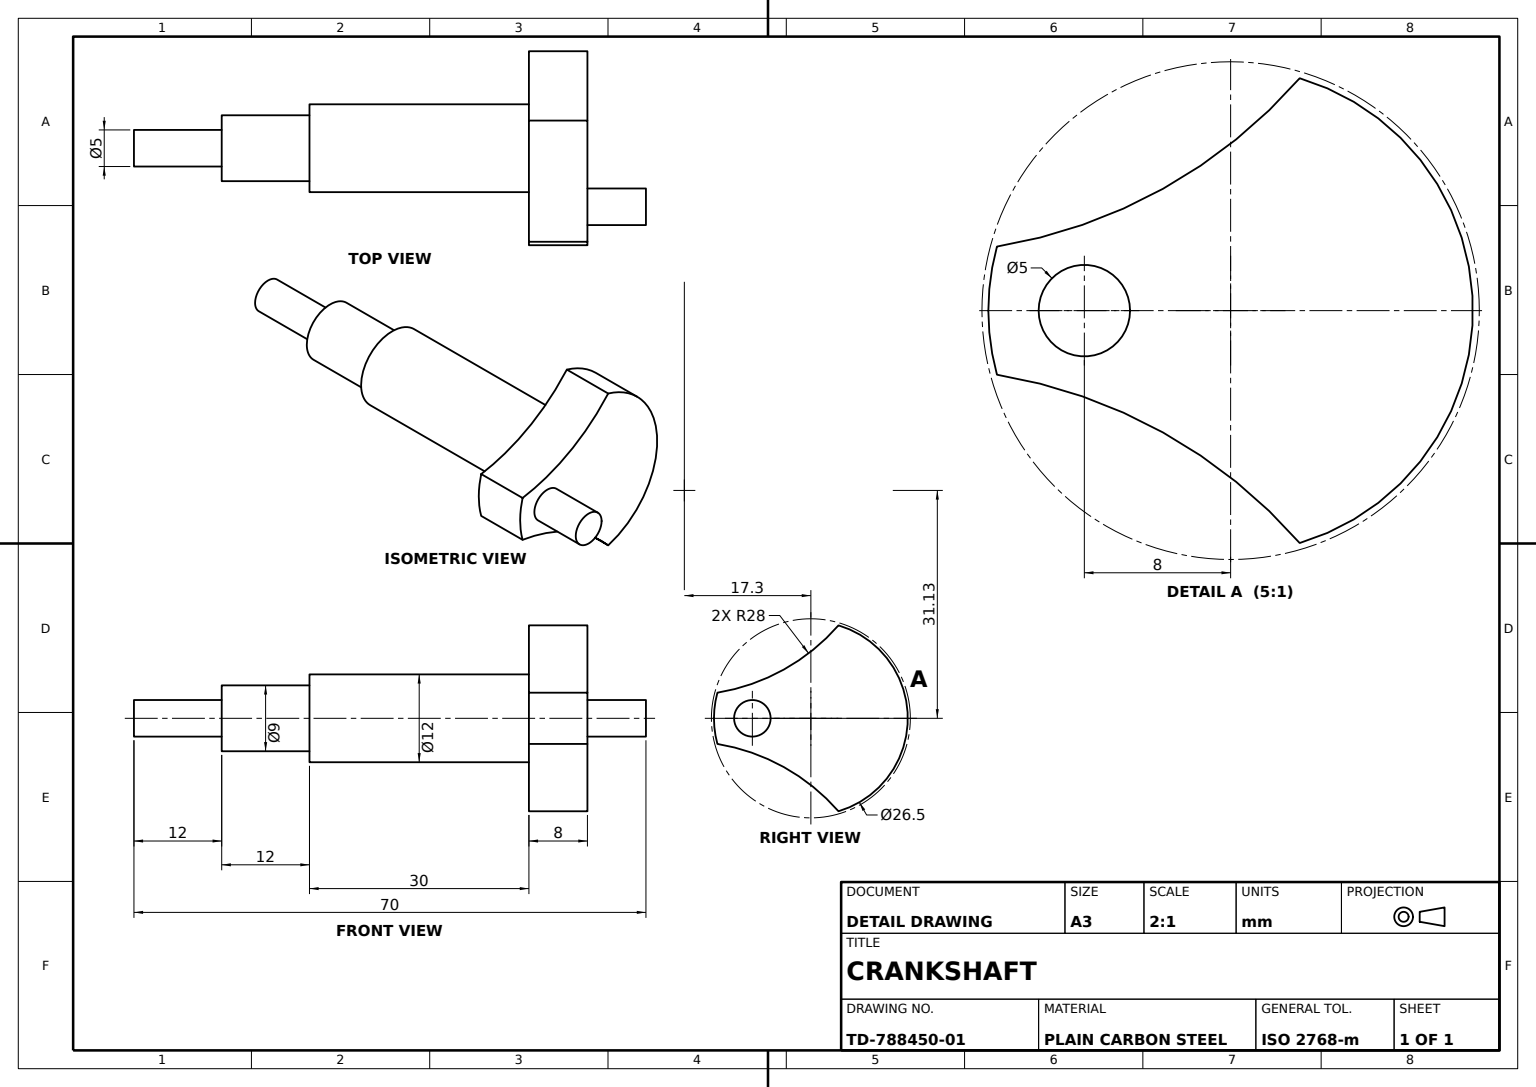
from build123d import *

# Parameters (mm, degrees)
MAIN_JOURNAL_PROFILE_12_R = 6
MAIN_JOURNAL_12_DEPTH     = 30
STEP_JOURNAL_PROFILE_9_R  = 4.5
STEP_JOURNAL_9_DEPTH      = 12
SHAFT_END_PROFILE_5_R     = 2.5
SHAFT_END_5_DEPTH         = 12
CRANK_WEB_DEPTH           = 8
CRANK_PIN_PROFILE_R       = 2.5
CRANK_PIN_DEPTH           = 8


with BuildPart() as part:
    # Main Journal Profile Ø12 → Main Journal Ø12 (new body)
    with BuildSketch(Plane.XY):
        Circle(MAIN_JOURNAL_PROFILE_12_R)
    extrude(amount=MAIN_JOURNAL_12_DEPTH)

    # Step Journal Profile Ø9 → Step Journal Ø9 (add)
    with BuildSketch(Plane.XY.offset(30)):
        Circle(STEP_JOURNAL_PROFILE_9_R)
    extrude(amount=STEP_JOURNAL_9_DEPTH)

    # Shaft End Profile Ø5 → Shaft End Ø5 (add)
    with BuildSketch(Plane.XY.offset(42)):
        Circle(SHAFT_END_PROFILE_5_R)
    extrude(amount=SHAFT_END_5_DEPTH)

    # Crank Web Profile → Crank Web (add)
    with BuildSketch(Plane(origin=(0, 0, 0), x_dir=(-1, 0, 0), z_dir=(0, 0, -1))):
        with BuildLine():
            ThreePointArc((-12.779377919, 3.5), (-13.25, 0), (-12.779377919, -3.5))
            ThreePointArc((-12.779377919, -3.5), (-3.699194839, -6.657412557), (3.777827997, -12.7000203))
            ThreePointArc((3.777827997, -12.7000203), (13.25, 0), (3.777827997, 12.7000203))
            ThreePointArc((3.777827997, 12.7000203), (-3.699194839, 6.657412557), (-12.779377919, 3.5))
        make_face()
    extrude(amount=CRANK_WEB_DEPTH)

    # Crank Pin Profile → Crank Pin (add)
    with BuildSketch(Plane(origin=(0, 0, -8), x_dir=(-1, 0, 0), z_dir=(0, 0, -1))):
        with Locations((-8, 0)):
            Circle(CRANK_PIN_PROFILE_R)
    extrude(amount=CRANK_PIN_DEPTH)


solid = part.part
